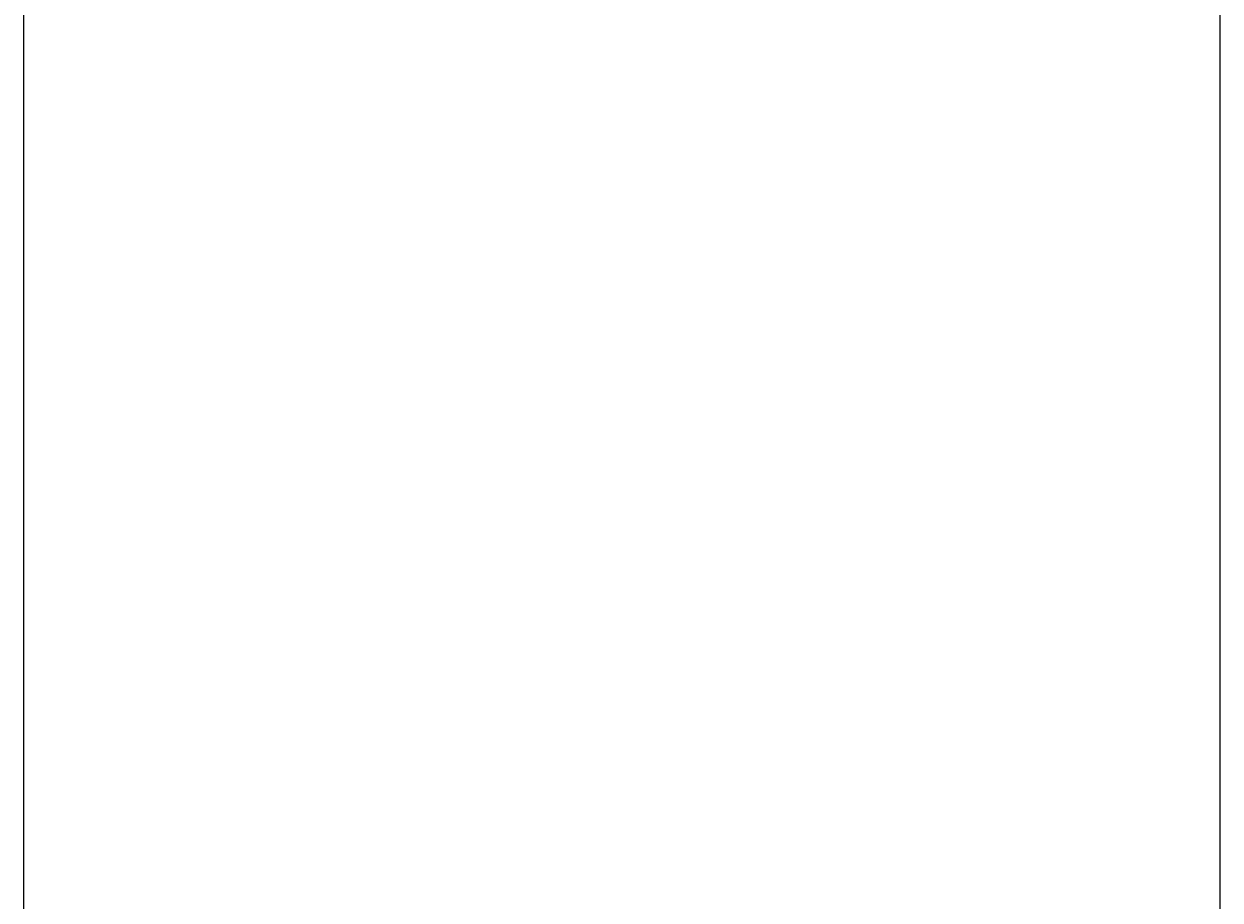
# Model space of a CAD drawing. Units: inches. Extents: x -61 to 1599, y -1316 to 257.
# Tile 133 of 204: x 372 to 456, y -77 to -16. Entities that reach past the tile are written whole.
import ezdxf

# ---------------------------------------------------------------- set-up
doc = ezdxf.new("R2010")
doc.units = ezdxf.units.IN
doc.header["$MEASUREMENT"] = 0
doc.layers.add('A-ANNO-DIMS', color=2, linetype='Continuous', lineweight=18)
doc.styles.get("Standard").update_dxf_attribs({"font": 'arial.ttf'})
doc.dimstyles.get("Standard").update_dxf_attribs({"dimtxt": 0.18, "dimasz": 0.18, "dimexe": 0.18, "dimexo": 0.0625, "dimgap": 0.09, "dimtad": 0, "dimtih": 1, "dimtoh": 1, "dimdec": 0, "dimzin": 0, "dimdsep": 46, "dimlunit": 3, "dimtxsty": 'Standard', "dimcen": 0.09, "dimadec": 0, "dimazin": 0, "dimtfac": 1, "dimtdec": 0, "dimtofl": 0, "dimtmove": 0, "dimatfit": 3, "dimfxl": 1, "dimtolj": 1, "dimtzin": 0, "dimarcsym": 0})

# ---------------------------------------------------------------- blocks, each defined once
blk = doc.blocks.new('*D703')
at = {"layer": 'A-ANNO-DIMS', "color": 0, "lineweight": -2, "transparency": 16777216}
for p, q in [((372.32, -616.882), (372.32, 257.457)), ((372.5, 257.277), (413.7, 257.277)), ((455.653, 257.277), (414.453, 257.277)), ((455.833, -616.882), (455.833, 257.457))]:
    blk.add_line(p, q, dxfattribs=at)
at = {"layer": 'A-ANNO-DIMS', "color": 0, "transparency": 16777216}
for points in [[(372.5, 257.307), (372.5, 257.247), (372.32, 257.277)], [(455.653, 257.307), (455.653, 257.247), (455.833, 257.277)]]:
    blk.add_solid(points, dxfattribs=at)
at = {"layer": 'DEFPOINTS', "color": 0, "transparency": 16777216}
for p in [(455.833, 257.277), (372.32, -616.945), (455.833, -616.945)]:
    blk.add_point(p, dxfattribs=at)
at = {"layer": 'A-ANNO-DIMS', "color": 0, "transparency": 16777216, "insert": (414.076, 257.277), "char_height": 0.18, "attachment_point": 5}
blk.add_mtext('\\A1;83.51', dxfattribs=at)

msp = doc.modelspace()

# ---------------------------------------------------------------- dimensions: what is measured, and where the dimension line sits
at = {"layer": 'A-ANNO-DIMS'}
dim = msp.add_linear_dim(base=(455.8327, 257.2771), p1=(372.3201, -616.9446), p2=(455.8327, -616.9446), dimstyle='Standard', override={"dimdec": 2, "dimlfac": 1, "dimrnd": 0, "dimzin": 0, "dimdsep": 46, "dimlunit": 2}, dxfattribs=at)
dim.commit()
dim.dimension.update_dxf_attribs({"geometry": '*D703', "text_midpoint": (414.0764, 257.2771)})

doc.saveas('drawing.dxf')
